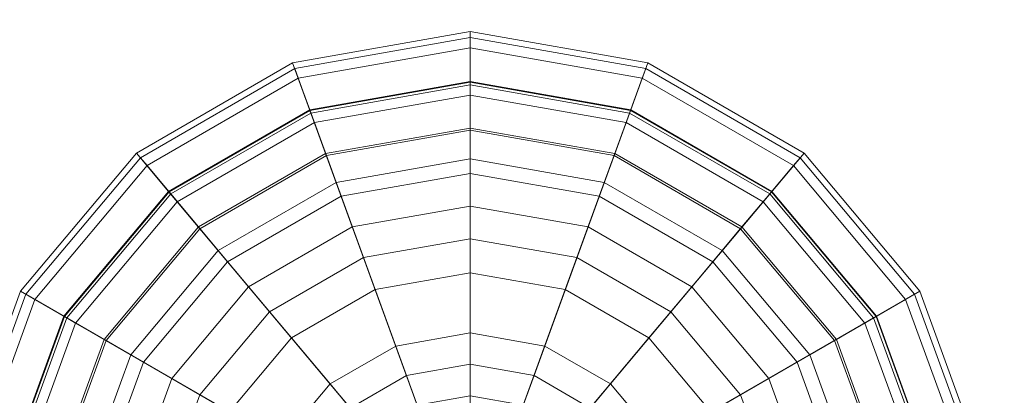
# Model space of a CAD drawing. Units: inches. Extents: x 375 to 1122, y 27 to 1069.
# Tile 50 of 155: x 720.906 to 723.474, y 310.871 to 311.85. Entities that reach past the tile are written whole.
import ezdxf

# ---------------------------------------------------------------- set-up
doc = ezdxf.new("R2010")
doc.units = ezdxf.units.IN
doc.layers.add('Furniture', color=30, linetype='Continuous', lineweight=18)

# ---------------------------------------------------------------- blocks, each defined once
blk = doc.blocks.new('A$C403C54AD')
at = {"linetype": 'ByBlock', "invisible_edges": 5}
for points in [[(0.818605, 0.976049, -0.033549), (0.847931, 0.959118, -0.024314), (0.86649, 1.028382, -0.024314), (0.832628, 1.028382, -0.033549)], [(0.847931, 0.959118, -0.019696), (0.831935, 0.968354, -0.019696), (0.84802, 1.028382, -0.019696), (0.86649, 1.028382, -0.019696)]]:
    blk.add_3dface(points, dxfattribs=at)
at = {"linetype": 'ByBlock'}
blk.add_3dface([(0.847931, 0.959118, -0.024314), (0.847931, 0.959118, -0.019696), (0.86649, 1.028382, -0.019696), (0.86649, 1.028382, -0.024314)], dxfattribs=at)
for points in [[(0.890422, 0.958466, -0.039553), (0.889855, 0.961682, -0.042784), (0.878804, 0.95766, -0.042784), (0.880436, 0.954832, -0.039553)], [(0.889855, 0.961682, -0.042784), (0.895735, 0.928335, -0.039705), (0.895735, 0.928335, -0.039705), (0.878804, 0.95766, -0.042784)], [(0.890429, 0.958426, 0.1202), (0.889924, 0.961289, 0.106976), (0.879003, 0.957315, 0.106976), (0.880457, 0.954797, 0.1202)], [(0.889924, 0.961289, 0.106976), (0.890041, 0.960625, 0.078734), (0.87934, 0.95673, 0.078734), (0.879003, 0.957315, 0.106976)], [(0.890041, 0.960625, 0.078734), (0.890973, 0.955342, 0.060725), (0.882023, 0.952084, 0.060725), (0.87934, 0.95673, 0.078734)], [(0.893266, 0.942333, -0.036278), (0.890422, 0.958466, -0.039553), (0.880436, 0.954832, -0.039553), (0.888627, 0.940645, -0.036278)], [(0.891296, 0.953506, 0.129606), (0.890429, 0.958426, 0.1202), (0.880457, 0.954797, 0.1202), (0.882955, 0.95047, 0.129606)], [(0.890459, 0.958252, 0.106759), (0.890947, 0.955485, 0.119395), (0.88195, 0.95221, 0.119395), (0.880545, 0.954643, 0.106759)], [(0.890574, 0.957604, 0.079219), (0.890459, 0.958252, 0.106759), (0.880545, 0.954643, 0.106759), (0.880874, 0.954073, 0.079219)], [(0.880436, 0.954832, -0.039553), (0.878804, 0.95766, -0.042784), (0.869795, 0.950101, -0.042784), (0.872296, 0.948002, -0.039553)], [(0.878804, 0.95766, -0.042784), (0.895735, 0.928335, -0.039705), (0.895735, 0.928335, -0.039705), (0.869795, 0.950101, -0.042784)], [(0.891461, 0.952574, 0.062072), (0.890574, 0.957604, 0.079219), (0.880874, 0.954073, 0.079219), (0.883428, 0.94965, 0.062072)], [(0.880457, 0.954797, 0.1202), (0.879003, 0.957315, 0.106976), (0.8701, 0.949844, 0.106976), (0.872327, 0.947976, 0.1202)], [(0.879003, 0.957315, 0.106976), (0.87934, 0.95673, 0.078734), (0.870617, 0.949411, 0.078734), (0.8701, 0.949844, 0.106976)], [(0.87934, 0.95673, 0.078734), (0.882023, 0.952084, 0.060725), (0.874727, 0.945962, 0.060725), (0.870617, 0.949411, 0.078734)], [(0.890947, 0.955485, 0.119395), (0.891831, 0.950474, 0.129606), (0.884494, 0.947804, 0.129606), (0.88195, 0.95221, 0.119395)], [(0.888627, 0.940645, -0.036278), (0.880436, 0.954832, -0.039553), (0.872296, 0.948002, -0.039553), (0.884846, 0.937471, -0.036278)], [(0.882955, 0.95047, 0.129606), (0.880457, 0.954797, 0.1202), (0.872327, 0.947976, 0.1202), (0.876155, 0.944764, 0.129606)], [(0.890973, 0.955342, 0.060725), (0.8922, 0.948383, 0.050493), (0.885556, 0.945965, 0.050493), (0.882023, 0.952084, 0.060725)], [(0.880545, 0.954643, 0.106759), (0.88195, 0.95221, 0.119395), (0.874615, 0.946056, 0.119395), (0.872463, 0.947862, 0.106759)], [(0.880874, 0.954073, 0.079219), (0.880545, 0.954643, 0.106759), (0.872463, 0.947862, 0.106759), (0.872967, 0.947439, 0.079219)], [(0.883428, 0.94965, 0.062072), (0.880874, 0.954073, 0.079219), (0.872967, 0.947439, 0.079219), (0.87688, 0.944156, 0.062072)], [(0.891831, 0.950474, 0.129606), (0.891296, 0.953506, 0.129606), (0.882955, 0.95047, 0.129606), (0.884494, 0.947804, 0.129606)], [(0.88195, 0.95221, 0.119395), (0.884494, 0.947804, 0.129606), (0.878513, 0.942785, 0.129606), (0.874615, 0.946056, 0.119395)], [(0.892587, 0.946186, 0.05268), (0.891461, 0.952574, 0.062072), (0.883428, 0.94965, 0.062072), (0.886671, 0.944033, 0.05268)], [(0.882023, 0.952084, 0.060725), (0.885556, 0.945965, 0.050493), (0.88014, 0.94142, 0.050493), (0.874727, 0.945962, 0.060725)], [(0.884494, 0.947804, 0.129606), (0.882955, 0.95047, 0.129606), (0.876155, 0.944764, 0.129606), (0.878513, 0.942785, 0.129606)], [(0.872296, 0.948002, -0.039553), (0.869795, 0.950101, -0.042784), (0.863915, 0.939916, -0.042784), (0.866983, 0.938799, -0.039553)], [(0.869795, 0.950101, -0.042784), (0.895735, 0.928335, -0.039705), (0.895735, 0.928335, -0.039705), (0.863915, 0.939916, -0.042784)], [(0.872327, 0.947976, 0.1202), (0.8701, 0.949844, 0.106976), (0.864289, 0.93978, 0.106976), (0.867021, 0.938785, 0.1202)], [(0.8701, 0.949844, 0.106976), (0.870617, 0.949411, 0.078734), (0.864924, 0.939549, 0.078734), (0.864289, 0.93978, 0.106976)], [(0.886671, 0.944033, 0.05268), (0.883428, 0.94965, 0.062072), (0.87688, 0.944156, 0.062072), (0.881848, 0.939987, 0.05268)], [(0.870617, 0.949411, 0.078734), (0.874727, 0.945962, 0.060725), (0.869965, 0.937714, 0.060725), (0.864924, 0.939549, 0.078734)], [(0.8922, 0.948383, 0.050493), (0.893978, 0.9383, 0.043125), (0.890675, 0.937098, 0.043125), (0.885556, 0.945965, 0.050493)], [(0.884846, 0.937471, -0.036278), (0.872296, 0.948002, -0.039553), (0.866983, 0.938799, -0.039553), (0.882378, 0.933196, -0.036278)], [(0.876155, 0.944764, 0.129606), (0.872327, 0.947976, 0.1202), (0.867021, 0.938785, 0.1202), (0.871716, 0.937076, 0.129606)], [(0.872463, 0.947862, 0.106759), (0.874615, 0.946056, 0.119395), (0.869828, 0.937764, 0.119395), (0.867188, 0.938725, 0.106759)], [(0.872967, 0.947439, 0.079219), (0.872463, 0.947862, 0.106759), (0.867188, 0.938725, 0.106759), (0.867806, 0.9385, 0.079219)], [(0.87688, 0.944156, 0.062072), (0.872967, 0.947439, 0.079219), (0.867806, 0.9385, 0.079219), (0.872606, 0.936753, 0.062072)], [(0.874615, 0.946056, 0.119395), (0.878513, 0.942785, 0.129606), (0.874609, 0.936024, 0.129606), (0.869828, 0.937764, 0.119395)], [(0.874727, 0.945962, 0.060725), (0.88014, 0.94142, 0.050493), (0.876605, 0.935297, 0.050493), (0.869965, 0.937714, 0.060725)], [(0.885556, 0.945965, 0.050493), (0.890675, 0.937098, 0.043125), (0.887983, 0.934839, 0.043125), (0.88014, 0.94142, 0.050493)], [(0.878513, 0.942785, 0.129606), (0.876155, 0.944764, 0.129606), (0.871716, 0.937076, 0.129606), (0.874609, 0.936024, 0.129606)], [(0.881848, 0.939987, 0.05268), (0.87688, 0.944156, 0.062072), (0.872606, 0.936753, 0.062072), (0.878701, 0.934534, 0.05268)], [(0.891283, 0.936046, 0.046044), (0.886671, 0.944033, 0.05268), (0.881848, 0.939987, 0.05268), (0.888914, 0.934058, 0.046044)], [(0.88014, 0.94142, 0.050493), (0.887983, 0.934839, 0.043125), (0.886226, 0.931795, 0.043125), (0.876605, 0.935297, 0.050493)], [(0.889651, 0.938871, -0.033413), (0.888627, 0.940645, -0.036278), (0.884846, 0.937471, -0.036278), (0.886415, 0.936155, -0.033413)], [(0.863915, 0.939916, -0.042784), (0.895735, 0.928335, -0.039705), (0.895735, 0.928335, -0.039705), (0.861872, 0.928335, -0.042784)], [(0.866983, 0.938799, -0.039553), (0.863915, 0.939916, -0.042784), (0.861872, 0.928335, -0.042784), (0.865138, 0.928335, -0.039553)], [(0.867021, 0.938785, 0.1202), (0.864289, 0.93978, 0.106976), (0.862271, 0.928335, 0.106976), (0.865179, 0.928335, 0.1202)], [(0.864289, 0.93978, 0.106976), (0.864924, 0.939549, 0.078734), (0.862946, 0.928335, 0.078734), (0.862271, 0.928335, 0.106976)], [(0.864924, 0.939549, 0.078734), (0.869965, 0.937714, 0.060725), (0.868311, 0.928335, 0.060725), (0.862946, 0.928335, 0.078734)], [(0.888914, 0.934058, 0.046044), (0.881848, 0.939987, 0.05268), (0.878701, 0.934534, 0.05268), (0.887368, 0.93138, 0.046044)], [(0.882378, 0.933196, -0.036278), (0.866983, 0.938799, -0.039553), (0.865138, 0.928335, -0.039553), (0.88152, 0.928335, -0.036278)], [(0.871716, 0.937076, 0.129606), (0.867021, 0.938785, 0.1202), (0.865179, 0.928335, 0.1202), (0.870175, 0.928335, 0.129606)], [(0.867188, 0.938725, 0.106759), (0.869828, 0.937764, 0.119395), (0.868166, 0.928335, 0.119395), (0.865356, 0.928335, 0.106759)], [(0.867806, 0.9385, 0.079219), (0.867188, 0.938725, 0.106759), (0.865356, 0.928335, 0.106759), (0.866014, 0.928335, 0.079219)], [(0.872606, 0.936753, 0.062072), (0.867806, 0.9385, 0.079219), (0.866014, 0.928335, 0.079219), (0.871122, 0.928335, 0.062072)], [(0.869828, 0.937764, 0.119395), (0.874609, 0.936024, 0.129606), (0.873253, 0.928335, 0.129606), (0.868166, 0.928335, 0.119395)], [(0.869965, 0.937714, 0.060725), (0.876605, 0.935297, 0.050493), (0.875377, 0.928335, 0.050493), (0.868311, 0.928335, 0.060725)], [(0.886415, 0.936155, -0.033413), (0.884846, 0.937471, -0.036278), (0.882378, 0.933196, -0.036278), (0.884302, 0.932496, -0.033413)], [(0.874609, 0.936024, 0.129606), (0.871716, 0.937076, 0.129606), (0.870175, 0.928335, 0.129606), (0.873253, 0.928335, 0.129606)], [(0.878701, 0.934534, 0.05268), (0.872606, 0.936753, 0.062072), (0.871122, 0.928335, 0.062072), (0.877607, 0.928335, 0.05268)], [(0.889552, 0.933523, -0.031367), (0.886415, 0.936155, -0.033413), (0.884302, 0.932496, -0.033413), (0.88815, 0.931095, -0.031367)], [(0.876605, 0.935297, 0.050493), (0.886226, 0.931795, 0.043125), (0.885616, 0.928335, 0.043125), (0.875377, 0.928335, 0.050493)], [(0.887368, 0.93138, 0.046044), (0.878701, 0.934534, 0.05268), (0.877607, 0.928335, 0.05268), (0.886831, 0.928335, 0.046044)], [(0.884302, 0.932496, -0.033413), (0.882378, 0.933196, -0.036278), (0.88152, 0.928335, -0.036278), (0.883568, 0.928335, -0.033413)], [(0.88815, 0.931095, -0.031367), (0.884302, 0.932496, -0.033413), (0.883568, 0.928335, -0.033413), (0.887664, 0.928335, -0.031367)], [(0.861872, 0.928335, -0.042784), (0.895735, 0.928335, -0.039705), (0.895735, 0.928335, -0.039705), (0.863915, 0.916753, -0.042784)], [(0.865138, 0.928335, -0.039553), (0.861872, 0.928335, -0.042784), (0.863915, 0.916753, -0.042784), (0.866983, 0.91787, -0.039553)], [(0.865179, 0.928335, 0.1202), (0.862271, 0.928335, 0.106976), (0.864289, 0.916889, 0.106976), (0.867021, 0.917884, 0.1202)], [(0.862271, 0.928335, 0.106976), (0.862946, 0.928335, 0.078734), (0.864924, 0.91712, 0.078734), (0.864289, 0.916889, 0.106976)], [(0.862946, 0.928335, 0.078734), (0.868311, 0.928335, 0.060725), (0.869965, 0.918955, 0.060725), (0.864924, 0.91712, 0.078734)], [(0.863915, 0.916753, -0.042784), (0.895735, 0.928335, -0.039705), (0.895735, 0.928335, -0.039705), (0.869795, 0.906568, -0.042784)], [(0.88152, 0.928335, -0.036278), (0.865138, 0.928335, -0.039553), (0.866983, 0.91787, -0.039553), (0.882378, 0.923473, -0.036278)], [(0.870175, 0.928335, 0.129606), (0.865179, 0.928335, 0.1202), (0.867021, 0.917884, 0.1202), (0.871716, 0.919593, 0.129606)], [(0.865356, 0.928335, 0.106759), (0.868166, 0.928335, 0.119395), (0.869828, 0.918905, 0.119395), (0.867188, 0.917944, 0.106759)], [(0.866014, 0.928335, 0.079219), (0.865356, 0.928335, 0.106759), (0.867188, 0.917944, 0.106759), (0.867806, 0.918169, 0.079219)], [(0.871122, 0.928335, 0.062072), (0.866014, 0.928335, 0.079219), (0.867806, 0.918169, 0.079219), (0.872606, 0.919916, 0.062072)], [(0.868166, 0.928335, 0.119395), (0.873253, 0.928335, 0.129606), (0.874609, 0.920646, 0.129606), (0.869828, 0.918905, 0.119395)], [(0.868311, 0.928335, 0.060725), (0.875377, 0.928335, 0.050493), (0.876605, 0.921372, 0.050493), (0.869965, 0.918955, 0.060725)], [(0.869795, 0.906568, -0.042784), (0.895735, 0.928335, -0.039705), (0.895735, 0.928335, -0.039705), (0.878804, 0.899009, -0.042784)], [(0.873253, 0.928335, 0.129606), (0.870175, 0.928335, 0.129606), (0.871716, 0.919593, 0.129606), (0.874609, 0.920646, 0.129606)], [(0.877607, 0.928335, 0.05268), (0.871122, 0.928335, 0.062072), (0.872606, 0.919916, 0.062072), (0.878701, 0.922135, 0.05268)], [(0.875377, 0.928335, 0.050493), (0.885616, 0.928335, 0.043125), (0.886226, 0.924874, 0.043125), (0.876605, 0.921372, 0.050493)], [(0.886831, 0.928335, 0.046044), (0.877607, 0.928335, 0.05268), (0.878701, 0.922135, 0.05268), (0.887368, 0.925289, 0.046044)], [(0.878804, 0.899009, -0.042784), (0.895735, 0.928335, -0.039705), (0.895735, 0.928335, -0.039705), (0.889855, 0.894987, -0.042784)], [(0.883568, 0.928335, -0.033413), (0.88152, 0.928335, -0.036278), (0.882378, 0.923473, -0.036278), (0.884302, 0.924173, -0.033413)], [(0.887664, 0.928335, -0.031367), (0.883568, 0.928335, -0.033413), (0.884302, 0.924173, -0.033413), (0.88815, 0.925574, -0.031367)], [(0.887368, 0.925289, 0.046044), (0.878701, 0.922135, 0.05268), (0.881848, 0.916683, 0.05268), (0.888914, 0.922611, 0.046044)], [(0.88815, 0.925574, -0.031367), (0.884302, 0.924173, -0.033413), (0.886415, 0.920514, -0.033413), (0.889552, 0.923147, -0.031367)], [(0.876605, 0.921372, 0.050493), (0.886226, 0.924874, 0.043125), (0.887983, 0.92183, 0.043125), (0.88014, 0.915249, 0.050493)], [(0.884302, 0.924173, -0.033413), (0.882378, 0.923473, -0.036278), (0.884846, 0.919198, -0.036278), (0.886415, 0.920514, -0.033413)], [(0.882378, 0.923473, -0.036278), (0.866983, 0.91787, -0.039553), (0.872296, 0.908668, -0.039553), (0.884846, 0.919198, -0.036278)], [(0.878701, 0.922135, 0.05268), (0.872606, 0.919916, 0.062072), (0.87688, 0.912514, 0.062072), (0.881848, 0.916683, 0.05268)], [(0.888914, 0.922611, 0.046044), (0.881848, 0.916683, 0.05268), (0.886671, 0.912636, 0.05268), (0.891283, 0.920623, 0.046044)], [(0.88014, 0.915249, 0.050493), (0.887983, 0.92183, 0.043125), (0.890675, 0.919571, 0.043125), (0.885556, 0.910704, 0.050493)], [(0.869965, 0.918955, 0.060725), (0.876605, 0.921372, 0.050493), (0.88014, 0.915249, 0.050493), (0.874727, 0.910707, 0.060725)], [(0.869828, 0.918905, 0.119395), (0.874609, 0.920646, 0.129606), (0.878513, 0.913884, 0.129606), (0.874615, 0.910614, 0.119395)], [(0.874609, 0.920646, 0.129606), (0.871716, 0.919593, 0.129606), (0.876155, 0.911905, 0.129606), (0.878513, 0.913884, 0.129606)], [(0.886415, 0.920514, -0.033413), (0.884846, 0.919198, -0.036278), (0.888627, 0.916025, -0.036278), (0.889651, 0.917798, -0.033413)], [(0.871716, 0.919593, 0.129606), (0.867021, 0.917884, 0.1202), (0.872327, 0.908694, 0.1202), (0.876155, 0.911905, 0.129606)], [(0.872606, 0.919916, 0.062072), (0.867806, 0.918169, 0.079219), (0.872967, 0.90923, 0.079219), (0.87688, 0.912514, 0.062072)], [(0.885556, 0.910704, 0.050493), (0.890675, 0.919571, 0.043125), (0.893978, 0.91837, 0.043125), (0.8922, 0.908286, 0.050493)], [(0.864924, 0.91712, 0.078734), (0.869965, 0.918955, 0.060725), (0.874727, 0.910707, 0.060725), (0.870617, 0.907259, 0.078734)], [(0.867188, 0.917944, 0.106759), (0.869828, 0.918905, 0.119395), (0.874615, 0.910614, 0.119395), (0.872463, 0.908807, 0.106759)], [(0.884846, 0.919198, -0.036278), (0.872296, 0.908668, -0.039553), (0.880436, 0.901837, -0.039553), (0.888627, 0.916025, -0.036278)], [(0.866983, 0.91787, -0.039553), (0.863915, 0.916753, -0.042784), (0.869795, 0.906568, -0.042784), (0.872296, 0.908668, -0.039553)], [(0.867021, 0.917884, 0.1202), (0.864289, 0.916889, 0.106976), (0.8701, 0.906825, 0.106976), (0.872327, 0.908694, 0.1202)], [(0.867806, 0.918169, 0.079219), (0.867188, 0.917944, 0.106759), (0.872463, 0.908807, 0.106759), (0.872967, 0.90923, 0.079219)], [(0.864289, 0.916889, 0.106976), (0.864924, 0.91712, 0.078734), (0.870617, 0.907259, 0.078734), (0.8701, 0.906825, 0.106976)], [(0.881848, 0.916683, 0.05268), (0.87688, 0.912514, 0.062072), (0.883428, 0.907019, 0.062072), (0.886671, 0.912636, 0.05268)], [(0.888627, 0.916025, -0.036278), (0.880436, 0.901837, -0.039553), (0.890422, 0.898203, -0.039553), (0.893266, 0.914336, -0.036278)], [(0.874727, 0.910707, 0.060725), (0.88014, 0.915249, 0.050493), (0.885556, 0.910704, 0.050493), (0.882023, 0.904585, 0.060725)], [(0.874615, 0.910614, 0.119395), (0.878513, 0.913884, 0.129606), (0.884494, 0.908865, 0.129606), (0.88195, 0.904459, 0.119395)], [(0.878513, 0.913884, 0.129606), (0.876155, 0.911905, 0.129606), (0.882955, 0.906199, 0.129606), (0.884494, 0.908865, 0.129606)], [(0.87688, 0.912514, 0.062072), (0.872967, 0.90923, 0.079219), (0.880874, 0.902596, 0.079219), (0.883428, 0.907019, 0.062072)], [(0.886671, 0.912636, 0.05268), (0.883428, 0.907019, 0.062072), (0.891461, 0.904095, 0.062072), (0.892587, 0.910483, 0.05268)], [(0.876155, 0.911905, 0.129606), (0.872327, 0.908694, 0.1202), (0.880457, 0.901872, 0.1202), (0.882955, 0.906199, 0.129606)], [(0.870617, 0.907259, 0.078734), (0.874727, 0.910707, 0.060725), (0.882023, 0.904585, 0.060725), (0.87934, 0.899939, 0.078734)], [(0.872463, 0.908807, 0.106759), (0.874615, 0.910614, 0.119395), (0.88195, 0.904459, 0.119395), (0.880545, 0.902026, 0.106759)], [(0.882023, 0.904585, 0.060725), (0.885556, 0.910704, 0.050493), (0.8922, 0.908286, 0.050493), (0.890973, 0.901327, 0.060725)], [(0.872967, 0.90923, 0.079219), (0.872463, 0.908807, 0.106759), (0.880545, 0.902026, 0.106759), (0.880874, 0.902596, 0.079219)], [(0.872296, 0.908668, -0.039553), (0.869795, 0.906568, -0.042784), (0.878804, 0.899009, -0.042784), (0.880436, 0.901837, -0.039553)], [(0.872327, 0.908694, 0.1202), (0.8701, 0.906825, 0.106976), (0.879003, 0.899355, 0.106976), (0.880457, 0.901872, 0.1202)], [(0.88195, 0.904459, 0.119395), (0.884494, 0.908865, 0.129606), (0.891831, 0.906195, 0.129606), (0.890947, 0.901184, 0.119395)], [(0.884494, 0.908865, 0.129606), (0.882955, 0.906199, 0.129606), (0.891296, 0.903163, 0.129606), (0.891831, 0.906195, 0.129606)], [(0.8701, 0.906825, 0.106976), (0.870617, 0.907259, 0.078734), (0.87934, 0.899939, 0.078734), (0.879003, 0.899355, 0.106976)], [(0.883428, 0.907019, 0.062072), (0.880874, 0.902596, 0.079219), (0.890574, 0.899065, 0.079219), (0.891461, 0.904095, 0.062072)], [(0.882955, 0.906199, 0.129606), (0.880457, 0.901872, 0.1202), (0.890429, 0.898243, 0.1202), (0.891296, 0.903163, 0.129606)], [(0.87934, 0.899939, 0.078734), (0.882023, 0.904585, 0.060725), (0.890973, 0.901327, 0.060725), (0.890041, 0.896044, 0.078734)], [(0.880545, 0.902026, 0.106759), (0.88195, 0.904459, 0.119395), (0.890947, 0.901184, 0.119395), (0.890459, 0.898417, 0.106759)], [(0.880874, 0.902596, 0.079219), (0.880545, 0.902026, 0.106759), (0.890459, 0.898417, 0.106759), (0.890574, 0.899065, 0.079219)], [(0.880436, 0.901837, -0.039553), (0.878804, 0.899009, -0.042784), (0.889855, 0.894987, -0.042784), (0.890422, 0.898203, -0.039553)], [(0.880457, 0.901872, 0.1202), (0.879003, 0.899355, 0.106976), (0.889924, 0.89538, 0.106976), (0.890429, 0.898243, 0.1202)], [(0.879003, 0.899355, 0.106976), (0.87934, 0.899939, 0.078734), (0.890041, 0.896044, 0.078734), (0.889924, 0.89538, 0.106976)]]:
    blk.add_3dface(points)

msp = doc.modelspace()

# ---------------------------------------------------------------- block references
at = {"layer": 'Furniture', "xscale": 39.9918517141215, "yscale": 39.9918517141215, "zscale": 39.9918517141215, "rotation": 270}
msp.add_blockref('A$C403C54AD', (684.9549, 346.2875, 0.024), dxfattribs=at)

doc.saveas('drawing.dxf')
